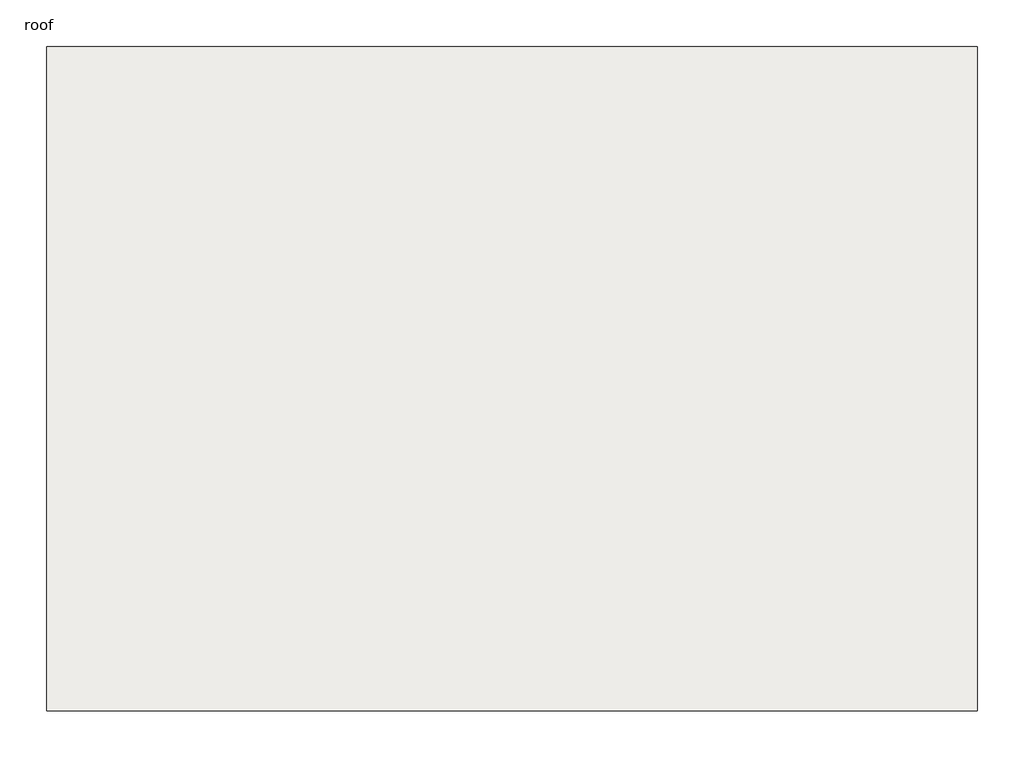
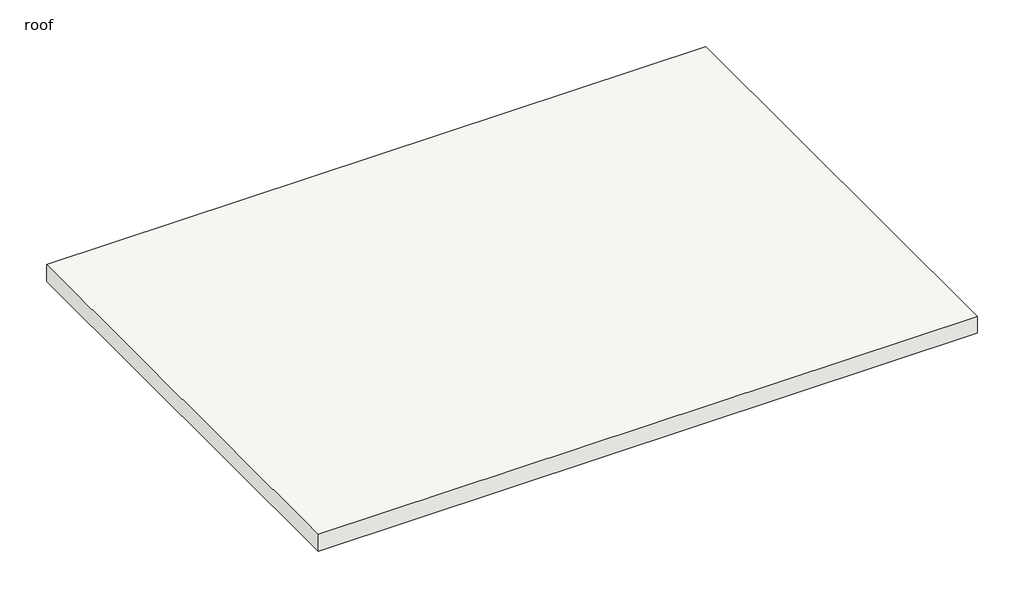
# One storey: 1 slab.
"""IFC4 building model written with IfcOpenShell, lengths in millimetres."""

from ifc_helpers import new_model, si_unit, frame, origin, place, context, project, spatial, polyline, outline, extrude, element, save

model = new_model("IFC4")

# Units and contexts
model_context = context("Model", 3, world=origin())
ifc_project = project(units=[si_unit("LENGTHUNIT", "METRE", prefix="MILLI")], contexts=[model_context])

# Site, building, storey
site = spatial("IfcSite", under=ifc_project)
building = spatial("IfcBuilding", under=site)
storey = spatial("IfcBuildingStorey", under=building, Name="roof", Elevation=9601.2)

# Slab
placement = place(None, origin())
element("IfcSlab", 1, ObjectType="6\"", at=placement, inside=storey, context=model_context, shape_type="SweptSolid", body=[
    extrude(outline(polyline([(5507.0585096, -332.3523906), (5507.0585096, -4396.3523906), (-182.5414904, -4396.3523906), (-182.5414904, -332.3523906), (5507.0585096, -332.3523906)])), frame((0.0, 0.0, 9448.8), z_axis=(0.0, 0.0, 1.0), x_axis=(1.0, 0.0, 0.0)), (0.0, 0.0, 1.0), 152.4),
])

save(model, "model.ifc")

# Revit data of these elements
# Type "6\""
#   Assembly Code = "B1010"
#   Function = 0
#   Layers, outside or top first: 0' - 6" no material (function 1)
# Element 1 (IfcSlab, "6\"")
#   Height Offset From Level = 0' - 0"
#   Phase Created = New Construction
#   Materials on its faces: "wall 2"
# Materials
#   "wall 2": class "Generic", colour RGB 34 30 27, transparency 0, Cost = 0
